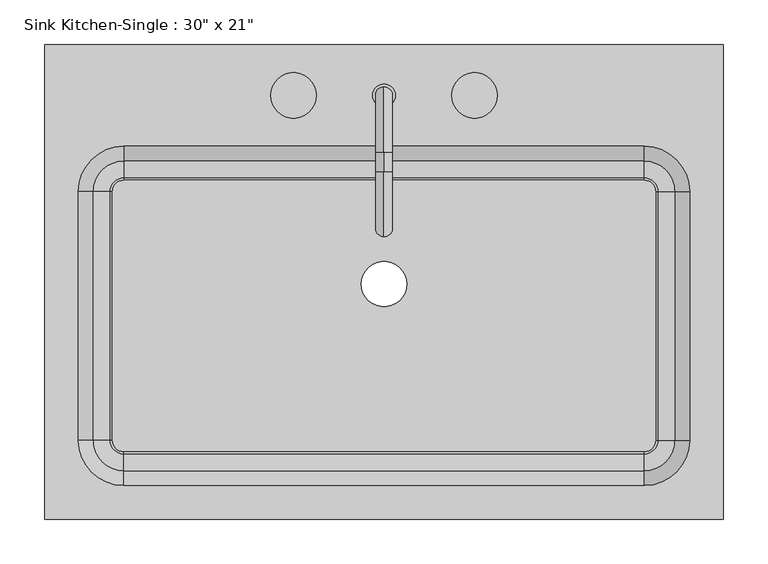
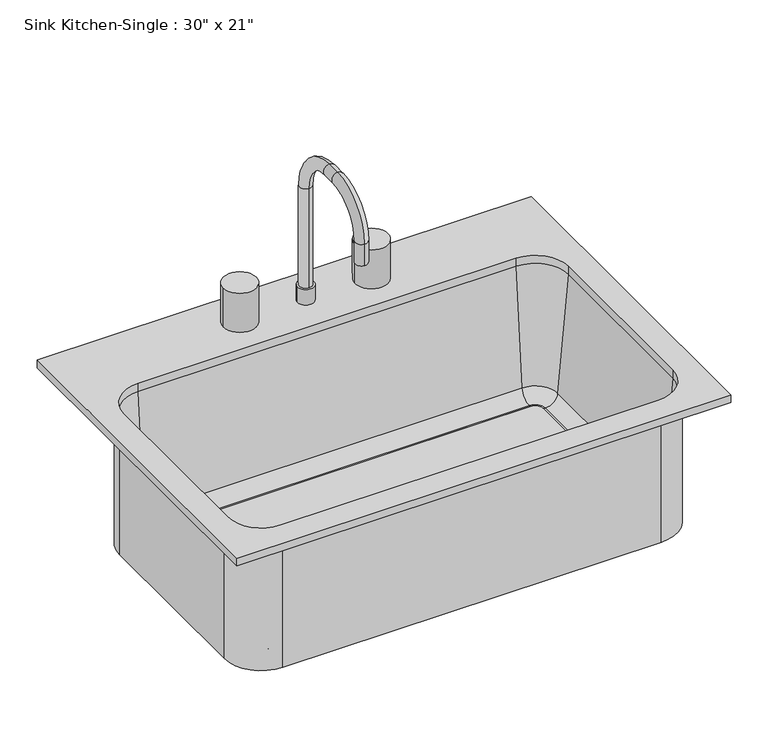
"""IFC4 building model written with IfcOpenShell, lengths in millimetres: flow terminal geometry."""

from ifc_helpers import new_model, si_unit, point, frame, frame_2d, origin, place, context, project, spatial, polyline, circle_curve, ellipse_curve, trimmed, segment, composite_curve, outline, extrude, source, transform, mapped, element, save
from ifc_brep_helpers import plane_surface, cylinder_surface, revolved_surface, advanced_brep


def flow_terminal_4d548711(model_context):
    return source(origin(), model_context, "Body", "SolidModel", [
        extrude(outline(composite_curve([segment(trimmed(circle_curve(frame_2d((307.7892406, 103.9454011)), 12.7), [point((307.7892406, 116.6454011))], [point((320.4892406, 103.9454011))], False, "CARTESIAN"), True, "CONTINUOUS"), segment(polyline([(320.4892406, 103.9454011), (320.4892406, -175.4545989)]), True, "CONTINUOUS"), segment(trimmed(circle_curve(frame_2d((307.7892406, -175.4545989)), 12.7), [point((320.4892406, -175.4545989))], [point((307.7892406, -188.1545989))], False, "CARTESIAN"), True, "CONTINUOUS"), segment(polyline([(307.7892406, -188.1545989), (-276.4107594, -188.1545989)]), True, "CONTINUOUS"), segment(trimmed(circle_curve(frame_2d((-276.4107594, -175.4545989)), 12.7), [point((-276.4107594, -188.1545989))], [point((-289.1107594, -175.4545989))], False, "CARTESIAN"), True, "CONTINUOUS"), segment(polyline([(-289.1107594, -175.4545989), (-289.1107594, 103.9454011)]), True, "CONTINUOUS"), segment(trimmed(circle_curve(frame_2d((-276.4107594, 103.9454011)), 12.7), [point((-289.1107594, 103.9454011))], [point((-276.4107594, 116.6454011))], False, "CARTESIAN"), True, "CONTINUOUS"), segment(polyline([(-276.4107594, 116.6454011), (307.7892406, 116.6454011)]), True, "CONTINUOUS")], self_intersect=False), holes=[composite_curve([segment(trimmed(circle_curve(frame_2d((15.6892406, 0.0)), 25.4), [point((-9.7107594, 0.0))], [point((41.0892406, 0.0))], True, "CARTESIAN"), True, "CONTINUOUS"), segment(trimmed(circle_curve(frame_2d((15.6892406, 0.0)), 25.4), [point((41.0892406, 0.0))], [point((-9.7107594, 0.0))], True, "CARTESIAN"), True, "CONTINUOUS")], self_intersect=False)]), frame((0.0, 0.0, 698.5), z_axis=(0.0, 0.0, 1.0), x_axis=(1.0, 0.0, 0.0)), (0.0, 0.0, 1.0), 9.525),
        extrude(outline(composite_curve([segment(trimmed(circle_curve(frame_2d((-85.9107594, 211.8954011)), 25.4), [point((-111.3107594, 211.8954011))], [point((-60.5107594, 211.8954011))], False, "CARTESIAN"), True, "CONTINUOUS"), segment(trimmed(circle_curve(frame_2d((-85.9107594, 211.8954011)), 25.4), [point((-60.5107594, 211.8954011))], [point((-111.3107594, 211.8954011))], False, "CARTESIAN"), True, "CONTINUOUS")], self_intersect=False)), frame((0.0, 0.0, 927.1), z_axis=(0.0, 0.0, 1.0), x_axis=(1.0, 0.0, 0.0)), (0.0, 0.0, 1.0), 63.5),
        extrude(outline(composite_curve([segment(trimmed(circle_curve(frame_2d((117.2892406, 211.8954011)), 25.4), [point((91.8892406, 211.8954011))], [point((142.6892406, 211.8954011))], False, "CARTESIAN"), True, "CONTINUOUS"), segment(trimmed(circle_curve(frame_2d((117.2892406, 211.8954011)), 25.4), [point((142.6892406, 211.8954011))], [point((91.8892406, 211.8954011))], False, "CARTESIAN"), True, "CONTINUOUS")], self_intersect=False)), frame((0.0, 0.0, 927.1), z_axis=(0.0, 0.0, 1.0), x_axis=(1.0, 0.0, 0.0)), (0.0, 0.0, 1.0), 63.5),
        advanced_brep(
        [(2.9892406, 211.8954011, 927.1), (28.3892406, 211.8954011, 927.1), (15.6892406, 221.4204011, 1114.425), (15.6892406, 202.3704011, 1114.425), (15.6892406, 202.3704011, 952.5), (15.6892406, 221.4204011, 952.5), (15.6892406, 148.3954011, 1187.45), (15.6892406, 148.3954011, 1168.4), (15.6892406, 126.1704011, 1187.45), (15.6892406, 126.1704011, 1168.4), (15.6892406, 53.1454011, 1114.425), (15.6892406, 72.1954011, 1114.425), (15.6892406, 53.1454011, 1079.5), (15.6892406, 72.1954011, 1079.5), (2.9892406, 211.8954011, 952.5), (28.3892406, 211.8954011, 952.5)],
        [
            (0, 1, circle_curve(frame((15.6892406, 211.8954011, 927.1), z_axis=(0.0, 0.0, -1.0), x_axis=(1.0, 0.0, 0.0)), 12.7)),
            (1, 0, circle_curve(frame((15.6892406, 211.8954011, 927.1), z_axis=(0.0, 0.0, -1.0), x_axis=(1.0, 0.0, 0.0)), 12.7)),
            (2, 3, circle_curve(frame((15.6892406, 211.8954011, 1114.425), z_axis=(0.0, 0.0, -1.0), x_axis=(0.0, -1.0, 0.0)), 9.525)),
            (3, 4),
            (4, 5, circle_curve(frame((15.6892406, 211.8954011, 952.5), z_axis=(0.0, 0.0, 1.0), x_axis=(0.0, -1.0, 0.0)), 9.525)),
            (5, 2),
            (3, 2, circle_curve(frame((15.6892406, 211.8954011, 1114.425), z_axis=(0.0, 0.0, -1.0), x_axis=(0.0, -1.0, 0.0)), 9.525)),
            (5, 4, circle_curve(frame((15.6892406, 211.8954011, 952.5), z_axis=(0.0, 0.0, 1.0), x_axis=(0.0, -1.0, 0.0)), 9.525)),
            (2, 6, circle_curve(frame((15.6892406, 148.3954011, 1114.425), z_axis=(1.0, 0.0, 0.0), x_axis=(0.0, 1.0, 0.0)), 73.025)),
            (6, 7, circle_curve(frame((15.6892406, 148.3954011, 1177.925), z_axis=(0.0, 1.0, 0.0), x_axis=(0.0, 0.0, -1.0)), 9.525)),
            (7, 3, circle_curve(frame((15.6892406, 148.3954011, 1114.425), z_axis=(-1.0, 0.0, 0.0), x_axis=(0.0, 1.0, 0.0)), 53.975)),
            (7, 6, circle_curve(frame((15.6892406, 148.3954011, 1177.925), z_axis=(0.0, 1.0, 0.0), x_axis=(0.0, 0.0, -1.0)), 9.525)),
            (6, 8),
            (8, 9, circle_curve(frame((15.6892406, 126.1704011, 1177.925), z_axis=(0.0, 1.0, 0.0), x_axis=(0.0, 0.0, -1.0)), 9.525)),
            (9, 7),
            (9, 8, circle_curve(frame((15.6892406, 126.1704011, 1177.925), z_axis=(0.0, 1.0, 0.0), x_axis=(0.0, 0.0, -1.0)), 9.525)),
            (8, 10, circle_curve(frame((15.6892406, 126.1704011, 1114.425), z_axis=(1.0, 0.0, 0.0), x_axis=(0.0, 0.0, 1.0)), 73.025)),
            (10, 11, circle_curve(frame((15.6892406, 62.6704011, 1114.425), z_axis=(0.0, 0.0, 1.0), x_axis=(0.0, 1.0, 0.0)), 9.525)),
            (11, 9, circle_curve(frame((15.6892406, 126.1704011, 1114.425), z_axis=(-1.0, 0.0, 0.0), x_axis=(0.0, 0.0, 1.0)), 53.975)),
            (11, 10, circle_curve(frame((15.6892406, 62.6704011, 1114.425), z_axis=(0.0, 0.0, 1.0), x_axis=(0.0, 1.0, 0.0)), 9.525)),
            (12, 13, circle_curve(frame((15.6892406, 62.6704011, 1079.5), z_axis=(0.0, 0.0, -1.0), x_axis=(0.0, 1.0, 0.0)), 9.525)),
            (13, 12, circle_curve(frame((15.6892406, 62.6704011, 1079.5), z_axis=(0.0, 0.0, -1.0), x_axis=(0.0, 1.0, 0.0)), 9.525)),
            (10, 12),
            (13, 11),
            (14, 15, circle_curve(frame((15.6892406, 211.8954011, 952.5), z_axis=(0.0, 0.0, 1.0), x_axis=(1.0, 0.0, 0.0)), 12.7)),
            (15, 14, circle_curve(frame((15.6892406, 211.8954011, 952.5), z_axis=(0.0, 0.0, 1.0), x_axis=(1.0, 0.0, 0.0)), 12.7)),
            (14, 0),
            (1, 15),
        ],
        [
            plane_surface(frame((15.6892406, 202.3704011, 927.1), z_axis=(0.0, 0.0, -1.0), x_axis=(1.0, 0.0, 0.0))),
            cylinder_surface(frame((15.6892406, 211.8954011, 927.1), z_axis=(0.0, 0.0, -1.0), x_axis=(0.0, -1.0, 0.0)), 9.525),
            revolved_surface(trimmed(ellipse_curve(frame((15.6892406, 211.8954011, 1114.425), z_axis=(0.0, 0.0, -1.0), x_axis=(0.0, -1.0, 0.0)), 9.525, 9.525), [point((15.6892406, 221.4204011, 1114.425))], [point((15.6892406, 202.3704011, 1114.425))], True, "CARTESIAN"), (15.6892406, 148.3954011, 1114.425), (1.0, 0.0, 0.0)),
            revolved_surface(trimmed(ellipse_curve(frame((15.6892406, 211.8954011, 1114.425), z_axis=(0.0, 0.0, -1.0), x_axis=(0.0, -1.0, 0.0)), 9.525, 9.525), [point((15.6892406, 202.3704011, 1114.425))], [point((15.6892406, 221.4204011, 1114.425))], True, "CARTESIAN"), (15.6892406, 148.3954011, 1114.425), (1.0, 0.0, 0.0)),
            cylinder_surface(frame((15.6892406, 148.3954011, 1177.925), z_axis=(0.0, 1.0, 0.0), x_axis=(0.0, 0.0, -1.0)), 9.525),
            revolved_surface(trimmed(ellipse_curve(frame((15.6892406, 126.1704011, 1177.925), z_axis=(0.0, 1.0, 0.0), x_axis=(0.0, 0.0, -1.0)), 9.525, 9.525), [point((15.6892406, 126.1704011, 1187.45))], [point((15.6892406, 126.1704011, 1168.4))], True, "CARTESIAN"), (15.6892406, 126.1704011, 1114.425), (1.0, 0.0, 0.0)),
            revolved_surface(trimmed(ellipse_curve(frame((15.6892406, 126.1704011, 1177.925), z_axis=(0.0, 1.0, 0.0), x_axis=(0.0, 0.0, -1.0)), 9.525, 9.525), [point((15.6892406, 126.1704011, 1168.4))], [point((15.6892406, 126.1704011, 1187.45))], True, "CARTESIAN"), (15.6892406, 126.1704011, 1114.425), (1.0, 0.0, 0.0)),
            plane_surface(frame((15.6892406, 53.1454011, 1079.5), z_axis=(0.0, 0.0, -1.0), x_axis=(-1.0, 0.0, 0.0))),
            cylinder_surface(frame((15.6892406, 62.6704011, 1114.425), z_axis=(0.0, 0.0, 1.0), x_axis=(0.0, 1.0, 0.0)), 9.525),
            plane_surface(frame((28.3892406, 211.8954011, 952.5), z_axis=(0.0, 0.0, 1.0), x_axis=(0.0, 1.0, 0.0))),
            cylinder_surface(frame((15.6892406, 211.8954011, 927.1), z_axis=(0.0, 0.0, 1.0), x_axis=(1.0, 0.0, 0.0)), 12.7),
        ],
        [
            (0, [[1, 2]]),
            (1, [[3, 4, 5, 6]]),
            (1, [[7, -6, 8, -4]]),
            (2, [[-3, 9, 10, 11]]),
            (3, [[-7, -11, 12, -9]]),
            (4, [[-10, 13, 14, 15]]),
            (4, [[-12, -15, 16, -13]]),
            (5, [[-14, 17, 18, 19]]),
            (6, [[-16, -19, 20, -17]]),
            (7, [[21, 22]]),
            (8, [[-18, 23, -22, 24]]),
            (8, [[-20, -24, -21, -23]]),
            (9, [[25, 26], [-5, -8]]),
            (10, [[-25, 27, -2, 28]]),
            (10, [[-26, -28, -1, -27]]),
        ],
    ),
        advanced_brep(
        [(396.6892406, 269.0454011, 927.1), (-365.3107594, 269.0454011, 927.1), (-365.3107594, -264.3545989, 927.1), (396.6892406, -264.3545989, 927.1), (307.7892406, 154.7454011, 927.1), (358.5892406, 103.9454011, 927.1), (358.5892406, -175.4545989, 927.1), (307.7892406, -226.2545989, 927.1), (-276.4107594, -226.2545989, 927.1), (-327.2107594, -175.4545989, 927.1), (-327.2107594, 103.9454011, 927.1), (-276.4107594, 154.7454011, 927.1), (396.6892406, 269.0454011, 914.4), (396.6892406, -264.3545989, 914.4), (-365.3107594, -264.3545989, 914.4), (-365.3107594, 269.0454011, 914.4), (364.9392406, 103.9454011, 914.4), (307.7892406, 161.0954011, 914.4), (-276.4107594, 161.0954011, 914.4), (-333.5607594, 103.9454011, 914.4), (-333.5607594, -175.4545989, 914.4), (-276.4107594, -232.6045989, 914.4), (307.7892406, -232.6045989, 914.4), (364.9392406, -175.4545989, 914.4), (307.7892406, 154.7454011, 914.4), (358.5892406, 103.9454011, 914.4), (358.5892406, -175.4545989, 914.4), (307.7892406, -226.2545989, 914.4), (-276.4107594, -226.2545989, 914.4), (-327.2107594, -175.4545989, 914.4), (-327.2107594, 103.9454011, 914.4), (-276.4107594, 154.7454011, 914.4), (364.9392406, 103.9454011, 698.5), (307.7892406, 161.0954011, 698.5), (320.4892406, 103.9454011, 698.5), (307.7892406, 116.6454011, 698.5), (320.4892406, 103.9454011, 708.025), (307.7892406, 116.6454011, 708.025), (323.0776588, 103.9454011, 708.025), (307.7892406, 119.2338193, 708.025), (342.0551678, 103.9454011, 725.4146831), (307.7892406, 138.2113283, 725.4146831), (364.9392406, -175.4545989, 698.5), (320.4892406, -175.4545989, 698.5), (320.4892406, -175.4545989, 708.025), (323.0776588, -175.4545989, 708.025), (342.0551678, -175.4545989, 725.4146831), (307.7892406, -232.6045989, 698.5), (307.7892406, -188.1545989, 698.5), (307.7892406, -188.1545989, 708.025), (307.7892406, -190.7430171, 708.025), (307.7892406, -209.7205261, 725.4146831), (-276.4107594, -232.6045989, 698.5), (-276.4107594, -188.1545989, 698.5), (-276.4107594, -188.1545989, 708.025), (-276.4107594, -190.7430171, 708.025), (-276.4107594, -209.7205261, 725.4146831), (-333.5607594, -175.4545989, 698.5), (-289.1107594, -175.4545989, 698.5), (-289.1107594, -175.4545989, 708.025), (-291.6991776, -175.4545989, 708.025), (-310.6766866, -175.4545989, 725.4146831), (-333.5607594, 103.9454011, 698.5), (-289.1107594, 103.9454011, 698.5), (-289.1107594, 103.9454011, 708.025), (-291.6991776, 103.9454011, 708.025), (-310.6766866, 103.9454011, 725.4146831), (-276.4107594, 161.0954011, 698.5), (-276.4107594, 116.6454011, 698.5), (-276.4107594, 116.6454011, 708.025), (-276.4107594, 119.2338193, 708.025), (-276.4107594, 138.2113283, 725.4146831)],
        [
            (0, 1),
            (1, 2),
            (2, 3),
            (3, 0),
            (4, 5, circle_curve(frame((307.7892406, 103.9454011, 927.1), z_axis=(0.0, 0.0, -1.0), x_axis=(1.0, 0.0, 0.0)), 50.8)),
            (5, 6),
            (6, 7, circle_curve(frame((307.7892406, -175.4545989, 927.1), z_axis=(0.0, 0.0, -1.0), x_axis=(1.0, 0.0, 0.0)), 50.8)),
            (7, 8),
            (8, 9, circle_curve(frame((-276.4107594, -175.4545989, 927.1), z_axis=(0.0, 0.0, -1.0), x_axis=(1.0, 0.0, 0.0)), 50.8)),
            (9, 10),
            (10, 11, circle_curve(frame((-276.4107594, 103.9454011, 927.1), z_axis=(0.0, 0.0, -1.0), x_axis=(1.0, 0.0, 0.0)), 50.8)),
            (11, 4),
            (12, 13),
            (13, 14),
            (14, 15),
            (15, 12),
            (16, 17, circle_curve(frame((307.7892406, 103.9454011, 914.4), z_axis=(0.0, 0.0, 1.0), x_axis=(0.0, 1.0, 0.0)), 57.15)),
            (17, 18),
            (18, 19, circle_curve(frame((-276.4107594, 103.9454011, 914.4), z_axis=(0.0, 0.0, 1.0), x_axis=(-1.0, 0.0, 0.0)), 57.15)),
            (19, 20),
            (20, 21, circle_curve(frame((-276.4107594, -175.4545989, 914.4), z_axis=(0.0, 0.0, 1.0), x_axis=(0.0, -1.0, 0.0)), 57.15)),
            (21, 22),
            (22, 23, circle_curve(frame((307.7892406, -175.4545989, 914.4), z_axis=(0.0, 0.0, 1.0), x_axis=(1.0, 0.0, 0.0)), 57.15)),
            (23, 16),
            (0, 12),
            (15, 1),
            (14, 2),
            (13, 3),
            (4, 24),
            (24, 25, circle_curve(frame((307.7892406, 103.9454011, 914.4), z_axis=(0.0, 0.0, -1.0), x_axis=(1.0, 0.0, 0.0)), 50.8)),
            (25, 5),
            (25, 26),
            (26, 6),
            (26, 27, circle_curve(frame((307.7892406, -175.4545989, 914.4), z_axis=(0.0, 0.0, -1.0), x_axis=(1.0, 0.0, 0.0)), 50.8)),
            (27, 7),
            (27, 28),
            (28, 8),
            (28, 29, circle_curve(frame((-276.4107594, -175.4545989, 914.4), z_axis=(0.0, 0.0, -1.0), x_axis=(1.0, 0.0, 0.0)), 50.8)),
            (29, 9),
            (29, 30),
            (30, 10),
            (30, 31, circle_curve(frame((-276.4107594, 103.9454011, 914.4), z_axis=(0.0, 0.0, -1.0), x_axis=(1.0, 0.0, 0.0)), 50.8)),
            (31, 11),
            (31, 24),
            (32, 33, circle_curve(frame((307.7892406, 103.9454011, 698.5), z_axis=(0.0, 0.0, 1.0), x_axis=(0.0, 1.0, 0.0)), 57.15)),
            (33, 17),
            (16, 32),
            (32, 34),
            (34, 35, circle_curve(frame((307.7892406, 103.9454011, 698.5), z_axis=(0.0, 0.0, 1.0), x_axis=(0.0, 1.0, 0.0)), 12.7)),
            (35, 33),
            (34, 36),
            (36, 37, circle_curve(frame((307.7892406, 103.9454011, 708.025), z_axis=(0.0, 0.0, 1.0), x_axis=(0.0, 1.0, 0.0)), 12.7)),
            (37, 35),
            (36, 38),
            (38, 39, circle_curve(frame((307.7892406, 103.9454011, 708.025), z_axis=(0.0, 0.0, 1.0), x_axis=(0.0, 1.0, 0.0)), 15.2884182)),
            (39, 37),
            (38, 40, circle_curve(frame((323.0776588, 103.9454011, 727.075), z_axis=(0.0, -1.0, 0.0), x_axis=(1.0, 0.0, 0.0)), 19.05)),
            (40, 41, circle_curve(frame((307.7892406, 103.9454011, 725.4146831), z_axis=(0.0, 0.0, 1.0), x_axis=(0.0, 1.0, 0.0)), 34.2659272)),
            (41, 39, circle_curve(frame((307.7892406, 119.2338193, 727.075), z_axis=(-1.0, 0.0, 0.0), x_axis=(0.0, 1.0, 0.0)), 19.05)),
            (40, 25),
            (24, 41),
            (23, 42),
            (42, 32),
            (42, 43),
            (43, 34),
            (43, 44),
            (44, 36),
            (44, 45),
            (45, 38),
            (45, 46, circle_curve(frame((323.0776588, -175.4545989, 727.075), z_axis=(0.0, -1.0, 0.0), x_axis=(1.0, 0.0, 0.0)), 19.05)),
            (46, 40),
            (46, 26),
            (22, 47),
            (47, 42, circle_curve(frame((307.7892406, -175.4545989, 698.5), z_axis=(0.0, 0.0, 1.0), x_axis=(1.0, 0.0, 0.0)), 57.15)),
            (47, 48),
            (48, 43, circle_curve(frame((307.7892406, -175.4545989, 698.5), z_axis=(0.0, 0.0, 1.0), x_axis=(1.0, 0.0, 0.0)), 12.7)),
            (48, 49),
            (49, 44, circle_curve(frame((307.7892406, -175.4545989, 708.025), z_axis=(0.0, 0.0, 1.0), x_axis=(1.0, 0.0, 0.0)), 12.7)),
            (49, 50),
            (50, 45, circle_curve(frame((307.7892406, -175.4545989, 708.025), z_axis=(0.0, 0.0, 1.0), x_axis=(1.0, 0.0, 0.0)), 15.2884182)),
            (50, 51, circle_curve(frame((307.7892406, -190.7430171, 727.075), z_axis=(-1.0, 0.0, 0.0), x_axis=(0.0, -1.0, 0.0)), 19.05)),
            (51, 46, circle_curve(frame((307.7892406, -175.4545989, 725.4146831), z_axis=(0.0, 0.0, 1.0), x_axis=(1.0, 0.0, 0.0)), 34.2659272)),
            (51, 27),
            (21, 52),
            (52, 47),
            (52, 53),
            (53, 48),
            (53, 54),
            (54, 49),
            (54, 55),
            (55, 50),
            (55, 56, circle_curve(frame((-276.4107594, -190.7430171, 727.075), z_axis=(-1.0, 0.0, 0.0), x_axis=(0.0, -1.0, 0.0)), 19.05)),
            (56, 51),
            (56, 28),
            (20, 57),
            (57, 52, circle_curve(frame((-276.4107594, -175.4545989, 698.5), z_axis=(0.0, 0.0, 1.0), x_axis=(0.0, -1.0, 0.0)), 57.15)),
            (57, 58),
            (58, 53, circle_curve(frame((-276.4107594, -175.4545989, 698.5), z_axis=(0.0, 0.0, 1.0), x_axis=(0.0, -1.0, 0.0)), 12.7)),
            (58, 59),
            (59, 54, circle_curve(frame((-276.4107594, -175.4545989, 708.025), z_axis=(0.0, 0.0, 1.0), x_axis=(0.0, -1.0, 0.0)), 12.7)),
            (59, 60),
            (60, 55, circle_curve(frame((-276.4107594, -175.4545989, 708.025), z_axis=(0.0, 0.0, 1.0), x_axis=(0.0, -1.0, 0.0)), 15.2884182)),
            (60, 61, circle_curve(frame((-291.6991776, -175.4545989, 727.075), z_axis=(0.0, 1.0, 0.0), x_axis=(-1.0, 0.0, 0.0)), 19.05)),
            (61, 56, circle_curve(frame((-276.4107594, -175.4545989, 725.4146831), z_axis=(0.0, 0.0, 1.0), x_axis=(0.0, -1.0, 0.0)), 34.2659272)),
            (61, 29),
            (19, 62),
            (62, 57),
            (62, 63),
            (63, 58),
            (63, 64),
            (64, 59),
            (64, 65),
            (65, 60),
            (65, 66, circle_curve(frame((-291.6991776, 103.9454011, 727.075), z_axis=(0.0, 1.0, 0.0), x_axis=(-1.0, 0.0, 0.0)), 19.05)),
            (66, 61),
            (66, 30),
            (18, 67),
            (67, 62, circle_curve(frame((-276.4107594, 103.9454011, 698.5), z_axis=(0.0, 0.0, 1.0), x_axis=(-1.0, 0.0, 0.0)), 57.15)),
            (67, 68),
            (68, 63, circle_curve(frame((-276.4107594, 103.9454011, 698.5), z_axis=(0.0, 0.0, 1.0), x_axis=(-1.0, 0.0, 0.0)), 12.7)),
            (68, 69),
            (69, 64, circle_curve(frame((-276.4107594, 103.9454011, 708.025), z_axis=(0.0, 0.0, 1.0), x_axis=(-1.0, 0.0, 0.0)), 12.7)),
            (69, 70),
            (70, 65, circle_curve(frame((-276.4107594, 103.9454011, 708.025), z_axis=(0.0, 0.0, 1.0), x_axis=(-1.0, 0.0, 0.0)), 15.2884182)),
            (70, 71, circle_curve(frame((-276.4107594, 119.2338193, 727.075), z_axis=(1.0, 0.0, 0.0), x_axis=(0.0, 1.0, 0.0)), 19.05)),
            (71, 66, circle_curve(frame((-276.4107594, 103.9454011, 725.4146831), z_axis=(0.0, 0.0, 1.0), x_axis=(-1.0, 0.0, 0.0)), 34.2659272)),
            (71, 31),
            (33, 67),
            (35, 68),
            (37, 69),
            (39, 70),
            (41, 71),
        ],
        [
            plane_surface(frame((-365.3107594, 269.0454011, 927.1), z_axis=(0.0, 0.0, 1.0), x_axis=(-1.0, 0.0, 0.0))),
            plane_surface(frame((-365.3107594, 269.0454011, 914.4), z_axis=(0.0, 0.0, -1.0), x_axis=(1.0, 0.0, 0.0))),
            plane_surface(frame((396.6892406, 269.0454011, 927.1), z_axis=(0.0, 1.0, 0.0), x_axis=(0.0, 0.0, -1.0))),
            plane_surface(frame((-365.3107594, 269.0454011, 927.1), z_axis=(-1.0, 0.0, 0.0), x_axis=(0.0, 0.0, -1.0))),
            plane_surface(frame((-365.3107594, -264.3545989, 927.1), z_axis=(0.0, -1.0, 0.0), x_axis=(0.0, 0.0, -1.0))),
            plane_surface(frame((396.6892406, -264.3545989, 927.1), z_axis=(1.0, 0.0, 0.0), x_axis=(0.0, 0.0, -1.0))),
            revolved_surface(polyline([(358.58924060000004, 103.9454011, 914.4), (358.58924060000004, 103.9454011, 927.1)]), (307.7892406, 103.9454011, 0.0), (0.0, 0.0, -1.0)),
            plane_surface(frame((358.5892406, 103.9454011, 927.1), z_axis=(-1.0, 0.0, 0.0), x_axis=(0.0, 0.0, -1.0))),
            revolved_surface(polyline([(358.58924060000004, -175.4545989, 914.4), (358.58924060000004, -175.4545989, 927.1)]), (307.7892406, -175.4545989, 0.0), (0.0, 0.0, -1.0)),
            plane_surface(frame((307.7892406, -226.2545989, 927.1), z_axis=(0.0, 1.0, 0.0), x_axis=(0.0, 0.0, -1.0))),
            revolved_surface(polyline([(-225.6107594, -175.4545989, 914.4), (-225.6107594, -175.4545989, 927.1)]), (-276.4107594, -175.4545989, 0.0), (0.0, 0.0, -1.0)),
            plane_surface(frame((-327.2107594, -175.4545989, 927.1), z_axis=(1.0, 0.0, 0.0), x_axis=(0.0, 0.0, -1.0))),
            revolved_surface(polyline([(-225.6107594, 103.9454011, 914.4), (-225.6107594, 103.9454011, 927.1)]), (-276.4107594, 103.9454011, 0.0), (0.0, 0.0, -1.0)),
            plane_surface(frame((-276.4107594, 154.7454011, 927.1), z_axis=(0.0, -1.0, 0.0), x_axis=(0.0, 0.0, -1.0))),
            cylinder_surface(frame((307.7892406, 103.9454011, 0.0), z_axis=(0.0, 0.0, -1.0), x_axis=(0.0, 1.0, 0.0)), 57.15),
            plane_surface(frame((307.7892406, 103.9454011, 698.5), z_axis=(0.0, 0.0, -1.0), x_axis=(0.0, 1.0, 0.0))),
            revolved_surface(polyline([(307.7892406, 116.6454011, 698.5), (307.7892406, 116.6454011, 708.025)]), (307.7892406, 103.9454011, 0.0), (0.0, 0.0, -1.0)),
            plane_surface(frame((307.7892406, 103.9454011, 708.025), z_axis=(0.0, 0.0, 1.0), x_axis=(0.0, 1.0, 0.0))),
            revolved_surface(trimmed(ellipse_curve(frame((307.7892406, 119.2338193, 727.075), z_axis=(1.0, 0.0, 0.0), x_axis=(0.0, 1.0, 0.0)), 19.05, 19.05), [point((307.7892406, 119.2338193, 708.025))], [point((307.7892406, 138.2113283, 725.4146831))], True, "CARTESIAN"), (307.7892406, 103.9454011, 0.0), (0.0, 0.0, -1.0)),
            revolved_surface(polyline([(307.7892406, 138.2113283, 725.4146831), (307.7892406, 154.7454011, 914.4)]), (307.7892406, 103.9454011, 0.0), (0.0, 0.0, -1.0)),
            plane_surface(frame((364.9392406, 103.9454011, 914.4), z_axis=(1.0, 0.0, 0.0), x_axis=(0.0, -1.0, 0.0))),
            plane_surface(frame((364.9392406, 103.9454011, 698.5), z_axis=(0.0, 0.0, -1.0), x_axis=(0.0, -1.0, 0.0))),
            plane_surface(frame((320.4892406, 103.9454011, 698.5), z_axis=(-1.0, 0.0, 0.0), x_axis=(0.0, -1.0, 0.0))),
            plane_surface(frame((320.4892406, 103.9454011, 708.025), z_axis=(0.0, 0.0, 1.0), x_axis=(0.0, -1.0, 0.0))),
            revolved_surface(polyline([(342.1276588, -175.45459889999998, 727.075), (342.1276588, 103.9454011, 727.075)]), (323.0776588, 103.9454011, 727.075), (0.0, -1.0, 0.0)),
            plane_surface(frame((342.0551678, 103.9454011, 725.4146831), z_axis=(-0.9961946980917442, 0.0, 0.08715574274767306), x_axis=(0.0, -1.0, 0.0))),
            cylinder_surface(frame((307.7892406, -175.4545989, 0.0), z_axis=(0.0, 0.0, -1.0), x_axis=(1.0, 0.0, 0.0)), 57.15),
            plane_surface(frame((307.7892406, -175.4545989, 698.5), z_axis=(0.0, 0.0, -1.0), x_axis=(1.0, 0.0, 0.0))),
            revolved_surface(polyline([(320.4892406, -175.4545989, 698.5), (320.4892406, -175.4545989, 708.025)]), (307.7892406, -175.4545989, 0.0), (0.0, 0.0, -1.0)),
            plane_surface(frame((307.7892406, -175.4545989, 708.025), z_axis=(0.0, 0.0, 1.0), x_axis=(1.0, 0.0, 0.0))),
            revolved_surface(trimmed(ellipse_curve(frame((323.0776588, -175.4545989, 727.075), z_axis=(0.0, -1.0, 0.0), x_axis=(1.0, 0.0, 0.0)), 19.05, 19.05), [point((323.0776588, -175.4545989, 708.025))], [point((342.0551678, -175.4545989, 725.4146831))], True, "CARTESIAN"), (307.7892406, -175.4545989, 0.0), (0.0, 0.0, -1.0)),
            revolved_surface(polyline([(342.0551678, -175.4545989, 725.4146831), (358.5892406, -175.4545989, 914.4)]), (307.7892406, -175.4545989, 0.0), (0.0, 0.0, -1.0)),
            plane_surface(frame((307.7892406, -232.6045989, 914.4), z_axis=(0.0, -1.0, 0.0), x_axis=(-1.0, 0.0, 0.0))),
            plane_surface(frame((307.7892406, -232.6045989, 698.5), z_axis=(0.0, 0.0, -1.0), x_axis=(-1.0, 0.0, 0.0))),
            plane_surface(frame((307.7892406, -188.1545989, 698.5), z_axis=(0.0, 1.0, 0.0), x_axis=(-1.0, 0.0, 0.0))),
            plane_surface(frame((307.7892406, -188.1545989, 708.025), z_axis=(0.0, 0.0, 1.0), x_axis=(-1.0, 0.0, 0.0))),
            revolved_surface(polyline([(-276.4107594, -209.79301710000001, 727.075), (307.7892406, -209.79301710000001, 727.075)]), (307.7892406, -190.7430171, 727.075), (-1.0, 0.0, 0.0)),
            plane_surface(frame((307.7892406, -209.7205261, 725.4146831), z_axis=(0.0, 0.9961946980917442, 0.08715574274767306), x_axis=(-1.0, 0.0, 0.0))),
            cylinder_surface(frame((-276.4107594, -175.4545989, 0.0), z_axis=(0.0, 0.0, -1.0), x_axis=(0.0, -1.0, 0.0)), 57.15),
            plane_surface(frame((-276.4107594, -175.4545989, 698.5), z_axis=(0.0, 0.0, -1.0), x_axis=(0.0, -1.0, 0.0))),
            revolved_surface(polyline([(-276.4107594, -188.1545989, 698.5), (-276.4107594, -188.1545989, 708.025)]), (-276.4107594, -175.4545989, 0.0), (0.0, 0.0, -1.0)),
            plane_surface(frame((-276.4107594, -175.4545989, 708.025), z_axis=(0.0, 0.0, 1.0), x_axis=(0.0, -1.0, 0.0))),
            revolved_surface(trimmed(ellipse_curve(frame((-276.4107594, -190.7430171, 727.075), z_axis=(-1.0, 0.0, 0.0), x_axis=(0.0, -1.0, 0.0)), 19.05, 19.05), [point((-276.4107594, -190.7430171, 708.025))], [point((-276.4107594, -209.7205261, 725.4146831))], True, "CARTESIAN"), (-276.4107594, -175.4545989, 0.0), (0.0, 0.0, -1.0)),
            revolved_surface(polyline([(-276.4107594, -209.7205261, 725.4146831), (-276.4107594, -226.2545989, 914.4)]), (-276.4107594, -175.4545989, 0.0), (0.0, 0.0, -1.0)),
            plane_surface(frame((-333.5607594, -175.4545989, 914.4), z_axis=(-1.0, 0.0, 0.0), x_axis=(0.0, 1.0, 0.0))),
            plane_surface(frame((-333.5607594, -175.4545989, 698.5), z_axis=(0.0, 0.0, -1.0), x_axis=(0.0, 1.0, 0.0))),
            plane_surface(frame((-289.1107594, -175.4545989, 698.5), z_axis=(1.0, 0.0, 0.0), x_axis=(0.0, 1.0, 0.0))),
            plane_surface(frame((-289.1107594, -175.4545989, 708.025), z_axis=(0.0, 0.0, 1.0), x_axis=(0.0, 1.0, 0.0))),
            revolved_surface(polyline([(-310.7491776, 103.94540109999997, 727.075), (-310.7491776, -175.4545989, 727.075)]), (-291.6991776, -175.4545989, 727.075), (0.0, 1.0, 0.0)),
            plane_surface(frame((-310.6766866, -175.4545989, 725.4146831), z_axis=(0.9961946980917442, 0.0, 0.08715574274767306), x_axis=(0.0, 1.0, 0.0))),
            cylinder_surface(frame((-276.4107594, 103.9454011, 0.0), z_axis=(0.0, 0.0, -1.0), x_axis=(-1.0, 0.0, 0.0)), 57.15),
            plane_surface(frame((-276.4107594, 103.9454011, 698.5), z_axis=(0.0, 0.0, -1.0), x_axis=(-1.0, 0.0, 0.0))),
            revolved_surface(polyline([(-289.1107594, 103.9454011, 698.5), (-289.1107594, 103.9454011, 708.025)]), (-276.4107594, 103.9454011, 0.0), (0.0, 0.0, -1.0)),
            plane_surface(frame((-276.4107594, 103.9454011, 708.025), z_axis=(0.0, 0.0, 1.0), x_axis=(-1.0, 0.0, 0.0))),
            revolved_surface(trimmed(ellipse_curve(frame((-291.6991776, 103.9454011, 727.075), z_axis=(0.0, 1.0, 0.0), x_axis=(-1.0, 0.0, 0.0)), 19.05, 19.05), [point((-291.6991776, 103.9454011, 708.025))], [point((-310.6766866, 103.9454011, 725.4146831))], True, "CARTESIAN"), (-276.4107594, 103.9454011, 0.0), (0.0, 0.0, -1.0)),
            revolved_surface(polyline([(-310.6766866, 103.9454011, 725.4146831), (-327.2107594, 103.9454011, 914.4)]), (-276.4107594, 103.9454011, 0.0), (0.0, 0.0, -1.0)),
            plane_surface(frame((-276.4107594, 161.0954011, 914.4), z_axis=(0.0, 1.0, 0.0), x_axis=(1.0, 0.0, 0.0))),
            plane_surface(frame((-276.4107594, 161.0954011, 698.5), z_axis=(0.0, 0.0, -1.0), x_axis=(1.0, 0.0, 0.0))),
            plane_surface(frame((-276.4107594, 116.6454011, 698.5), z_axis=(0.0, -1.0, 0.0), x_axis=(1.0, 0.0, 0.0))),
            plane_surface(frame((-276.4107594, 116.6454011, 708.025), z_axis=(0.0, 0.0, 1.0), x_axis=(1.0, 0.0, 0.0))),
            revolved_surface(polyline([(307.7892406, 138.2838193, 727.075), (-276.4107594, 138.2838193, 727.075)]), (-276.4107594, 119.2338193, 727.075), (1.0, 0.0, 0.0)),
            plane_surface(frame((-276.4107594, 138.2113283, 725.4146831), z_axis=(0.0, -0.9961946980917442, 0.08715574274767306), x_axis=(1.0, 0.0, 0.0))),
        ],
        [
            (0, [[1, 2, 3, 4], [5, 6, 7, 8, 9, 10, 11, 12]]),
            (1, [[13, 14, 15, 16], [17, 18, 19, 20, 21, 22, 23, 24]]),
            (2, [[-1, 25, -16, 26]]),
            (3, [[-2, -26, -15, 27]]),
            (4, [[-3, -27, -14, 28]]),
            (5, [[-4, -28, -13, -25]]),
            (6, [[-5, 29, 30, 31]]),
            (7, [[-6, -31, 32, 33]]),
            (8, [[-7, -33, 34, 35]]),
            (9, [[-8, -35, 36, 37]]),
            (10, [[-9, -37, 38, 39]]),
            (11, [[-10, -39, 40, 41]]),
            (12, [[-11, -41, 42, 43]]),
            (13, [[-12, -43, 44, -29]]),
            (14, [[45, 46, -17, 47]]),
            (15, [[-45, 48, 49, 50]]),
            (16, [[-49, 51, 52, 53]]),
            (17, [[-52, 54, 55, 56]]),
            (18, [[-55, 57, 58, 59]]),
            (19, [[-58, 60, -30, 61]]),
            (20, [[-47, -24, 62, 63]]),
            (21, [[-48, -63, 64, 65]]),
            (22, [[-51, -65, 66, 67]]),
            (23, [[-54, -67, 68, 69]]),
            (24, [[-57, -69, 70, 71]]),
            (25, [[-60, -71, 72, -32]]),
            (26, [[-62, -23, 73, 74]]),
            (27, [[-64, -74, 75, 76]]),
            (28, [[-66, -76, 77, 78]]),
            (29, [[-68, -78, 79, 80]]),
            (30, [[-70, -80, 81, 82]]),
            (31, [[-72, -82, 83, -34]]),
            (32, [[-73, -22, 84, 85]]),
            (33, [[-75, -85, 86, 87]]),
            (34, [[-77, -87, 88, 89]]),
            (35, [[-79, -89, 90, 91]]),
            (36, [[-81, -91, 92, 93]]),
            (37, [[-83, -93, 94, -36]]),
            (38, [[-84, -21, 95, 96]]),
            (39, [[-86, -96, 97, 98]]),
            (40, [[-88, -98, 99, 100]]),
            (41, [[-90, -100, 101, 102]]),
            (42, [[-92, -102, 103, 104]]),
            (43, [[-94, -104, 105, -38]]),
            (44, [[-95, -20, 106, 107]]),
            (45, [[-97, -107, 108, 109]]),
            (46, [[-99, -109, 110, 111]]),
            (47, [[-101, -111, 112, 113]]),
            (48, [[-103, -113, 114, 115]]),
            (49, [[-105, -115, 116, -40]]),
            (50, [[-106, -19, 117, 118]]),
            (51, [[-108, -118, 119, 120]]),
            (52, [[-110, -120, 121, 122]]),
            (53, [[-112, -122, 123, 124]]),
            (54, [[-114, -124, 125, 126]]),
            (55, [[-116, -126, 127, -42]]),
            (56, [[-46, 128, -117, -18]]),
            (57, [[-50, 129, -119, -128]]),
            (58, [[-53, 130, -121, -129]]),
            (59, [[-56, 131, -123, -130]]),
            (60, [[-59, 132, -125, -131]]),
            (61, [[-61, -44, -127, -132]]),
        ],
    ),
    ])


if __name__ == "__main__":
    model = new_model("IFC4")
    model_context = context("Model", 3, world=origin())
    ifc_project = project(units=[si_unit("LENGTHUNIT", "METRE", prefix="MILLI")], contexts=[model_context])
    site = spatial("IfcSite", under=ifc_project)
    building = spatial("IfcBuilding", under=site)
    placement = place(None, origin())
    flow_terminal_shape = flow_terminal_4d548711(model_context)
    element("IfcFlowTerminal", 1, ObjectType="Sink Kitchen-Single : 30\" x 21\"", at=placement, inside=building, context=model_context, shape_type="MappedRepresentation", body=[
        mapped(flow_terminal_shape, transform((0.0, 0.0, 0.0), x_axis=(1.0, 0.0, 0.0), y_axis=(0.0, 1.0, 0.0), z_axis=(0.0, 0.0, 1.0))),
    ])
    save(model, "model.ifc")

# Revit data of these elements
# Type "Sink Kitchen-Single : 30\" x 21\""
#   Assembly Code = "D2010410"
#   Counter Height = 3' - 0"
#   Depth = 1' - 9"
#   Width = 2' - 6"
#   Faucet Material = Steel, Polished
#   Sink Material = Steel, Polished
#   Default Elevation = 0
# Element 1 (IfcFlowTerminal, "Sink Kitchen-Single : 30\" x 21\"")
#   Materials on its faces: "Steel, Polished"
# Materials
#   "Steel, Polished": class "Metal", colour RGB 192 192 192, transparency 0, Description = "Polished steel", Cost = 0
